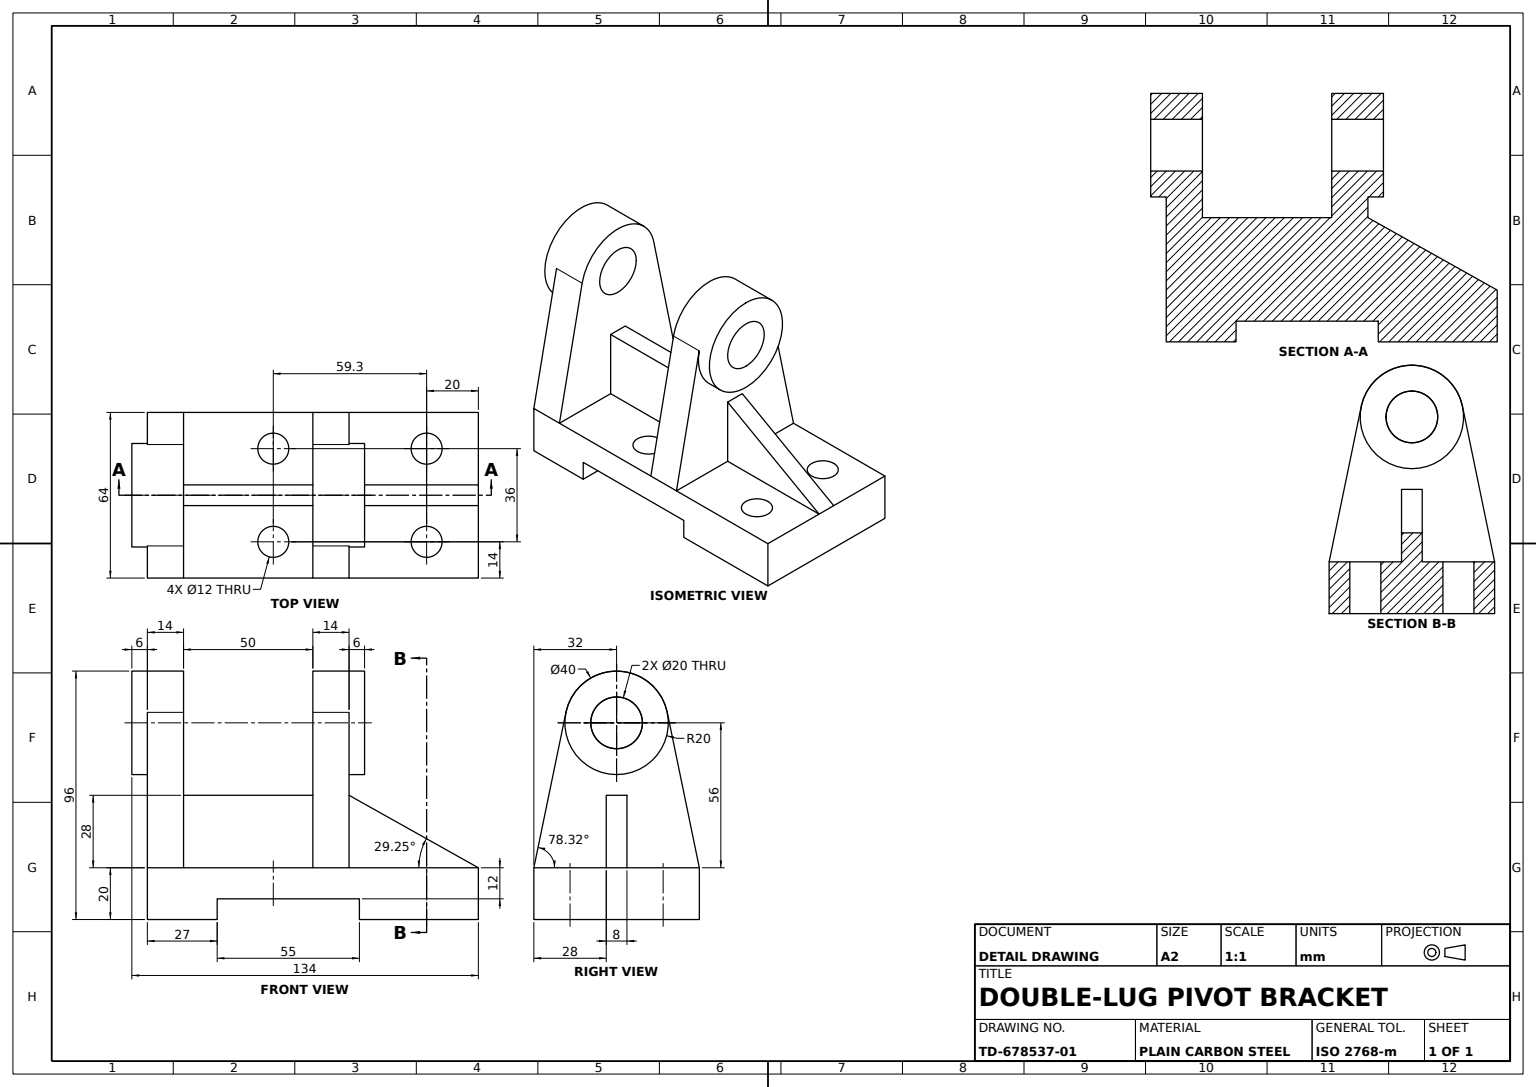
from build123d import *

# Parameters (mm, degrees)
BASE_PLATE_DEPTH        = 64
CLEVIS_LUG_1_DEPTH      = 14
LUG_START               = 6
LUG_1_HUB_SKETCH_R      = 20
LUG_1_HUB_BOSS_40_DEPTH = 6
LUG_1_PIN_BORE_SKETCH_R = 10
LUG_1_PIN_BORE_20_DEPTH = 30
WEB_BLOCK_SKETCH_W      = 50
WEB_BLOCK_SKETCH_H      = 28
WEB_BLOCK_DEPTH         = 64
WEB_TRIM_CUT_1_SKETCH_W = 50
WEB_TRIM_CUT_1_SKETCH_H = 28
WEB_TRIM_CUT_1_DEPTH    = 28
WEB_TRIM_CUT_2_SKETCH_W = 50
WEB_TRIM_CUT_2_SKETCH_H = 28
WEB_TRIM_CUT_2_DEPTH    = 28
CLEVIS_LUG_2_DEPTH      = 14
LUG_2_HUB_SKETCH_R      = 20
LUG_2_HUB_BOSS_40_DEPTH = 6
LUG_START_2             = -30
LUG_2_PIN_BORE_SKETCH_R = 10
LUG_2_PIN_BORE_20_DEPTH = 30
GUSSET_BLOCK_DEPTH      = 64
GUSSET_TRIM_CUT_1_DEPTH = 28
GUSSET_TRIM_CUT_2_DEPTH = 28
MOUNTING_HOLES_SKETCH_R = 6
MOUNTING_HOLES_12_DEPTH = 28


with BuildPart() as part:
    # Base Plate Profile Sketch → Base Plate (new body)
    with BuildSketch(Plane.XY):
        Polygon((0, 0), (27, 0), (82, 0), (128, 0), (128, -20), (82, -20), (82, -12), (27, -12), (27, -20), (0, -20), align=None)
    extrude(amount=-BASE_PLATE_DEPTH)

    # Clevis Lug 1 Sketch → Clevis Lug 1 (add)
    with BuildSketch(Plane.ZY):
        with BuildLine():
            Line((-51.585841233, 60.049052133), (-64, 0))
            Line((-64, 0), (-32, 0))
            Line((-32, 0), (0, 0))
            Line((0, 0), (-12.414158767, 60.049052133))
            ThreePointArc((-12.414158767, 60.049052133), (-32, 76), (-51.585841233, 60.049052133))
        make_face()
    extrude(amount=-CLEVIS_LUG_1_DEPTH)

    # Lug 1 Hub Sketch → Lug 1 Hub Boss Ø40 (add)
    with BuildSketch(Plane.ZY.offset(LUG_START)):
        with Locations((-32, 56)):
            Circle(LUG_1_HUB_SKETCH_R)
    extrude(amount=-LUG_1_HUB_BOSS_40_DEPTH)

    # Lug 1 Pin Bore Sketch → Lug 1 Pin Bore Ø20 (cut)
    with BuildSketch(Plane.ZY.offset(6)):
        with Locations((-32, 56)):
            Circle(LUG_1_PIN_BORE_SKETCH_R)
    extrude(amount=-LUG_1_PIN_BORE_20_DEPTH, mode=Mode.SUBTRACT)

    # Web Block Sketch → Web Block (add)
    with BuildSketch(Plane.XY):
        with Locations((39, 14)):
            Rectangle(WEB_BLOCK_SKETCH_W, WEB_BLOCK_SKETCH_H)
    extrude(amount=-WEB_BLOCK_DEPTH)

    # Web Trim Cut 1 Sketch → Web Trim Cut 1 (cut)
    with BuildSketch(Plane.XY):
        with Locations((39, 14)):
            Rectangle(WEB_TRIM_CUT_1_SKETCH_W, WEB_TRIM_CUT_1_SKETCH_H)
    extrude(amount=-WEB_TRIM_CUT_1_DEPTH, mode=Mode.SUBTRACT)

    # Web Trim Cut 2 Sketch → Web Trim Cut 2 (cut)
    with BuildSketch(Plane(origin=(0, 0, -64), x_dir=(-1, 0, 0), z_dir=(0, 0, -1))):
        with Locations((-39, 14)):
            Rectangle(WEB_TRIM_CUT_2_SKETCH_W, WEB_TRIM_CUT_2_SKETCH_H)
    extrude(amount=-WEB_TRIM_CUT_2_DEPTH, mode=Mode.SUBTRACT)

    # Clevis Lug 2 Sketch → Clevis Lug 2 (add)
    with BuildSketch(Plane(origin=(64, 0, 0), x_dir=(0, 0, -1), z_dir=(1, 0, 0))):
        with BuildLine():
            Line((0, 0), (12.414158767, 60.049052133))
            ThreePointArc((12.414158767, 60.049052133), (32, 76), (51.585841233, 60.049052133))
            Line((51.585841233, 60.049052133), (64, 0))
            Line((64, 0), (0, 0))
        make_face()
    extrude(amount=CLEVIS_LUG_2_DEPTH)

    # Lug 2 Hub Sketch → Lug 2 Hub Boss Ø40 (add)
    with BuildSketch(Plane(origin=(78, 0, 0), x_dir=(0, 0, -1), z_dir=(1, 0, 0))):
        with Locations(Location((32, 56, 0), (0, 0, 180))):
            Circle(LUG_2_HUB_SKETCH_R)
    extrude(amount=LUG_2_HUB_BOSS_40_DEPTH)

    # Lug 2 Pin Bore Sketch → Lug 2 Pin Bore Ø20 (cut)
    with BuildSketch(Plane(origin=(84, 0, 0), x_dir=(0, 0, -1), z_dir=(1, 0, 0)).offset(LUG_START_2)):
        with Locations(Location((32, 56, 0), (0, 0, 180))):
            Circle(LUG_2_PIN_BORE_SKETCH_R)
    extrude(amount=LUG_2_PIN_BORE_20_DEPTH, mode=Mode.SUBTRACT)

    # Gusset Block Sketch → Gusset Block (add)
    with BuildSketch(Plane.XY):
        Polygon((78, 0), (78, 28), (128, 0), align=None)
    extrude(amount=-GUSSET_BLOCK_DEPTH)

    # Gusset Trim Cut 1 Sketch → Gusset Trim Cut 1 (cut)
    with BuildSketch(Plane.XY):
        Polygon((78, 28), (78, 0), (128, 0), align=None)
    extrude(amount=-GUSSET_TRIM_CUT_1_DEPTH, mode=Mode.SUBTRACT)

    # Gusset Trim Cut 2 Sketch → Gusset Trim Cut 2 (cut)
    with BuildSketch(Plane(origin=(0, 0, -64), x_dir=(-1, 0, 0), z_dir=(0, 0, -1))):
        Polygon((-128, 0), (-78, 0), (-78, 28), align=None)
    extrude(amount=-GUSSET_TRIM_CUT_2_DEPTH, mode=Mode.SUBTRACT)

    # Mounting Holes Sketch → Mounting Holes Ø12 (cut)
    with BuildSketch(Plane(origin=(0, 0, 0), x_dir=(1, 0, 0), z_dir=(0, 1, 0))):
        with Locations(Location((48.7, 50, 0), (0, 0, 270))):
            Circle(MOUNTING_HOLES_SKETCH_R)
        with Locations(Location((108, 50, 0), (0, 0, 270))):
            Circle(MOUNTING_HOLES_SKETCH_R)
        with Locations(Location((108, 14, 0), (0, 0, 270))):
            Circle(MOUNTING_HOLES_SKETCH_R)
        with Locations(Location((48.7, 14, 0), (0, 0, 270))):
            Circle(MOUNTING_HOLES_SKETCH_R)
    extrude(amount=-MOUNTING_HOLES_12_DEPTH, mode=Mode.SUBTRACT)


solid = part.part
